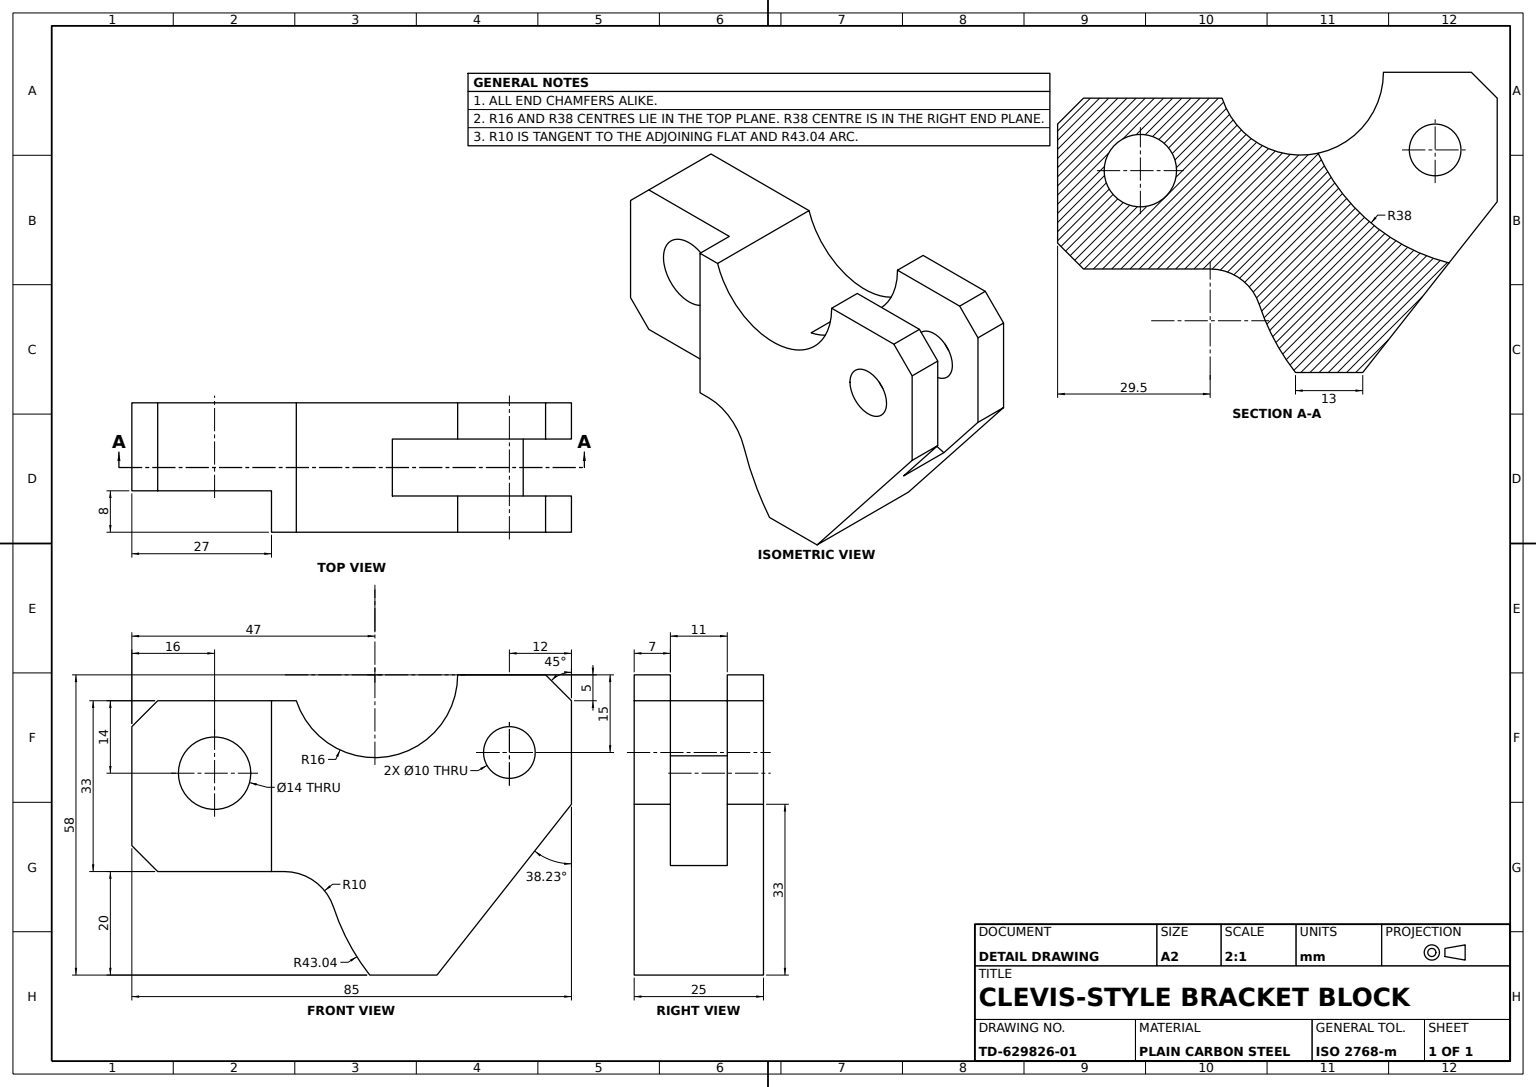
from build123d import *

# Parameters (mm, degrees)
BRACKET_PROFILE_SKETCH_R   = 7
BRACKET_PROFILE_SKETCH_R_2 = 5
BRACKET_BODY_25MM_DEPTH    = 12.5
EDGE_CHAMFER_5MM_SIZE      = 5
SLOT_SKETCH_W              = 27
SLOT_SKETCH_H              = 33
SLOT_CUT_8MM_DEPTH         = 8
CROSS_HOLE_SKETCH_R        = 38
CROSS_HOLE_CUT_DEPTH       = 5.5


with BuildPart() as part:
    # Bracket Profile Sketch → Bracket Body 25mm (new, symmetric)
    with BuildSketch(Plane.XY):
        with BuildLine():
            Line((16, -3.84), (38, -3.84))
            Line((38, -3.84), (38, -28.84))
            Line((38, -28.84), (12, -61.84))
            Line((12, -61.84), (-1, -61.84))
            ThreePointArc((-1, -61.84), (-5.071476538, -55.587008251), (-8.001806768, -48.724793466))
            ThreePointArc((-8.001806768, -48.724793466), (-11.637006424, -43.74209702), (-17.504200585, -41.84))
            Line((-17.504200585, -41.84), (-47, -41.84))
            Line((-47, -41.84), (-47, -8.84))
            Line((-47, -8.84), (-15.198684154, -8.84))
            ThreePointArc((-15.198684154, -8.84), (2.531901809, -19.638400971), (16, -3.84))
        make_face()
        with Locations((-31, -22.84)):
            Circle(BRACKET_PROFILE_SKETCH_R, mode=Mode.SUBTRACT)
        with Locations((26, -18.84)):
            Circle(BRACKET_PROFILE_SKETCH_R_2, mode=Mode.SUBTRACT)
    extrude(amount=BRACKET_BODY_25MM_DEPTH, both=True)

    # Edge Chamfer 5mm
    edge_chamfer_5mm_edges = [part.edges().sort_by_distance(p)[0] for p in [
        (38, -3.84, 0),
        (-47, -41.84, 0),
        (-47, -8.84, 0),
    ]]
    chamfer(edge_chamfer_5mm_edges, length=EDGE_CHAMFER_5MM_SIZE)

    # Slot Sketch → Slot Cut 8mm (cut)
    with BuildSketch(Plane.XY.offset(12.5)):
        with Locations((-33.5, -25.34)):
            Rectangle(SLOT_SKETCH_W, SLOT_SKETCH_H)
    extrude(amount=-SLOT_CUT_8MM_DEPTH, mode=Mode.SUBTRACT)

    # Cross Hole Sketch → Cross Hole Cut (cut, symmetric)
    with BuildSketch(Plane.XY):
        with Locations((38, -3.84)):
            Circle(CROSS_HOLE_SKETCH_R)
    extrude(amount=CROSS_HOLE_CUT_DEPTH, both=True, mode=Mode.SUBTRACT)


solid = part.part
